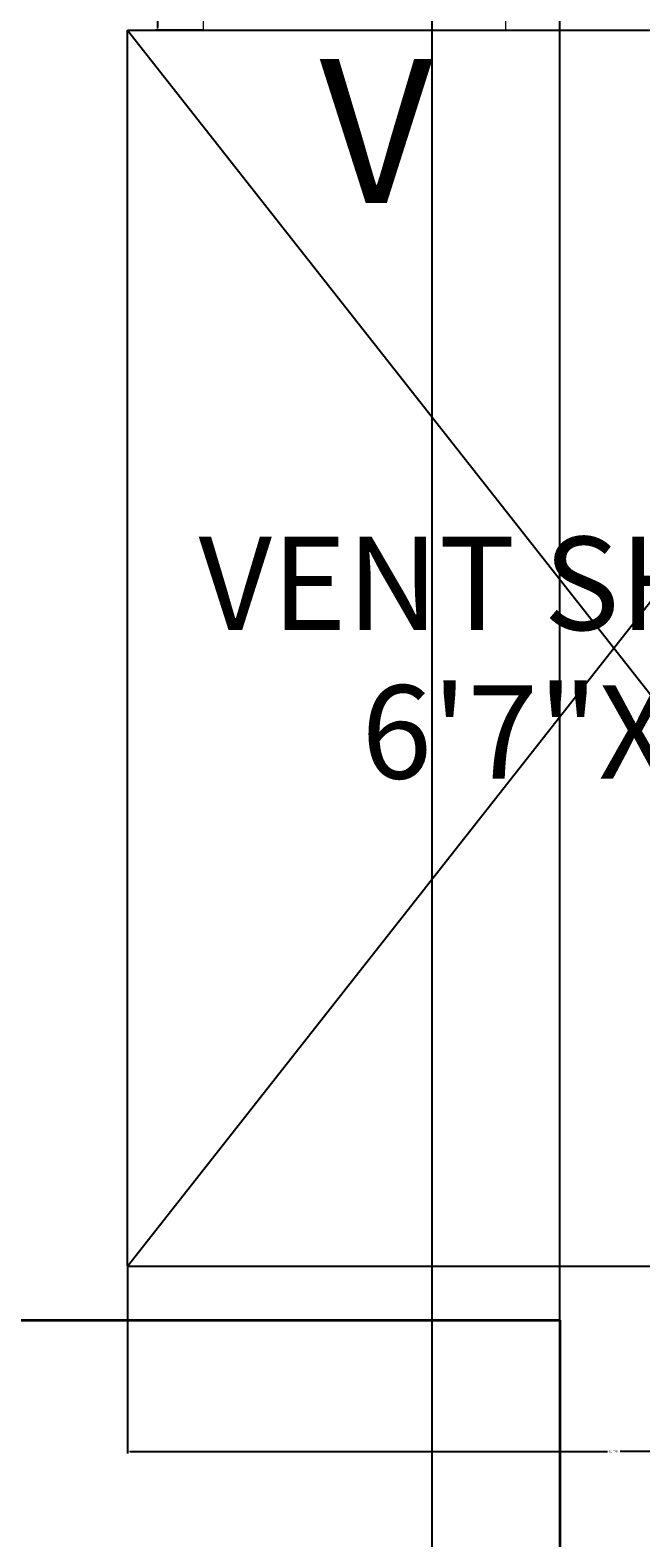
# Model space of a CAD drawing. Units: feet. Extents: x 5816 to 6644, y 25475 to 26788.
# Tile 16 of 23: x 6181 to 6232, y 26373 to 26499. Entities that reach past the tile are written whole.
import ezdxf

# ---------------------------------------------------------------- set-up
doc = ezdxf.new("R2010")
doc.units = ezdxf.units.FT
for name, color, linetype, lineweight in [('A-ANNO-DIMS', 2, 'Continuous', 13), ('A-ANNO-TEXT', 7, 'Continuous', 18), ('A-AREA-IDEN', 7, 'Continuous', 18), ('A-FLOR-SHFT', 8, 'Continuous', 25), ('A-GLAZ', 4, 'Continuous', 18), ('A-WALL', 7, 'Continuous', 35)]:
    doc.layers.add(name, color=color, linetype=linetype, lineweight=lineweight)
doc.styles.get("Standard").update_dxf_attribs({"font": 'arial.ttf'})
doc.dimstyles.get("Standard").update_dxf_attribs({"dimtxt": 0.18, "dimasz": 0.18, "dimexe": 0.18, "dimexo": 0.0625, "dimgap": 0.09, "dimtad": 0, "dimtih": 1, "dimtoh": 1, "dimdec": 4, "dimzin": 0, "dimdsep": 46, "dimtxsty": 'Standard', "dimcen": 0.09, "dimadec": 0, "dimazin": 0, "dimtfac": 1, "dimtdec": 4, "dimtofl": 0, "dimtmove": 0, "dimatfit": 3, "dimfxl": 1, "dimtolj": 1, "dimtzin": 0, "dimarcsym": 0})

# ---------------------------------------------------------------- blocks, each defined once
blk = doc.blocks.new('WIN-VENT-WIDE')
for p, q in [((0, 0), (0, -9)), ((25.2, 0), (25.2, -9)), ((0, -4.5), (25.2, -4.5))]:
    blk.add_line(p, q)
blk = doc.blocks.new('VENT-SHAFT')
for p, q in [((0, 0), (0, 103)), ((0, 103), (81, 103)), ((0, 103), (81, 0)), ((0, 0), (81, 103)), ((81, 103), (45, 103)), ((81, 0), (81, 103)), ((0, 0), (81, 0)), ((81, 0), (45, 0))]:
    blk.add_line(p, q)
blk = doc.blocks.new('*D50')
at = {"layer": 'A-ANNO-DIMS', "color": 0, "lineweight": -2, "transparency": 16777216}
for p, q in [((6195.53, 26507.58), (6191.64, 26507.58)), ((6191.82, 26507.4), (6191.82, 26503.27)), ((6191.82, 26498.76), (6191.82, 26502.9)), ((6195.53, 26498.58), (6191.64, 26498.58))]:
    blk.add_line(p, q, dxfattribs=at)
at = {"layer": 'A-ANNO-DIMS', "color": 0, "transparency": 16777216}
for points in [[(6191.79, 26507.4), (6191.85, 26507.4), (6191.82, 26507.58)], [(6191.79, 26498.76), (6191.85, 26498.76), (6191.82, 26498.58)]]:
    blk.add_solid(points, dxfattribs=at)
at = {"layer": 'Defpoints', "color": 0, "transparency": 16777216}
for p in [(6191.82, 26507.58), (6195.6, 26507.58), (6195.6, 26498.58)]:
    blk.add_point(p, dxfattribs=at)
at = {"layer": 'A-ANNO-DIMS', "color": 0, "transparency": 16777216, "insert": (6191.82, 26503.08), "char_height": 0.18, "attachment_point": 5}
blk.add_mtext('\\A1;9 TYP.', dxfattribs=at)
blk = doc.blocks.new('*D54')
at = {"layer": 'A-ANNO-DIMS', "color": 0, "lineweight": -2, "transparency": 16777216}
for p, q in [((6189.31, 26395.52), (6189.31, 26379.95)), ((6270.31, 26395.52), (6270.31, 26379.95)), ((6189.49, 26380.13), (6229.28, 26380.13)), ((6270.13, 26380.13), (6230.34, 26380.13))]:
    blk.add_line(p, q, dxfattribs=at)
at = {"layer": 'A-ANNO-DIMS', "color": 0, "transparency": 16777216}
for points in [[(6189.49, 26380.16), (6189.49, 26380.1), (6189.31, 26380.13)], [(6270.13, 26380.16), (6270.13, 26380.1), (6270.31, 26380.13)]]:
    blk.add_solid(points, dxfattribs=at)
at = {"layer": 'Defpoints', "color": 0, "transparency": 16777216}
for p in [(6189.31, 26395.58), (6270.31, 26395.58), (6270.31, 26380.13)]:
    blk.add_point(p, dxfattribs=at)
at = {"layer": 'A-ANNO-DIMS', "color": 0, "transparency": 16777216, "insert": (6229.81, 26380.13), "char_height": 0.18, "attachment_point": 5}
blk.add_mtext('\\A1;81 TYP.', dxfattribs=at)
blk = doc.blocks.new('*D60')
at = {"layer": 'A-ANNO-DIMS', "color": 0, "lineweight": -2, "transparency": 16777216}
for p, q in [((6106.98, 26094.4), (6106.98, 26787.91)), ((6107.16, 26787.73), (6224.93, 26787.73)), ((6343.5, 26787.73), (6225.72, 26787.73)), ((6343.68, 26094.4), (6343.68, 26787.91))]:
    blk.add_line(p, q, dxfattribs=at)
at = {"layer": 'A-ANNO-DIMS', "color": 0, "transparency": 16777216}
for points in [[(6107.16, 26787.76), (6107.16, 26787.7), (6106.98, 26787.73)], [(6343.5, 26787.76), (6343.5, 26787.7), (6343.68, 26787.73)]]:
    blk.add_solid(points, dxfattribs=at)
at = {"layer": 'Defpoints', "color": 0, "transparency": 16777216}
for p in [(6343.68, 26787.73), (6106.98, 26094.34), (6343.68, 26094.34)]:
    blk.add_point(p, dxfattribs=at)
at = {"layer": 'A-ANNO-DIMS', "color": 0, "transparency": 16777216, "insert": (6225.33, 26787.73), "char_height": 0.18, "attachment_point": 5}
blk.add_mtext('\\A1;236.7', dxfattribs=at)
blk = doc.blocks.new('*D72')
at = {"layer": 'A-ANNO-DIMS', "color": 0, "lineweight": -2, "transparency": 16777216}
for p, q in [((6214.69, 26168.65), (6214.69, 26787.91)), ((6214.87, 26787.73), (6219.56, 26787.73)), ((6225.13, 26787.73), (6220.44, 26787.73)), ((6225.31, 26177.65), (6225.31, 26787.91))]:
    blk.add_line(p, q, dxfattribs=at)
at = {"layer": 'A-ANNO-DIMS', "color": 0, "transparency": 16777216}
for points in [[(6214.87, 26787.76), (6214.87, 26787.7), (6214.69, 26787.73)], [(6225.13, 26787.76), (6225.13, 26787.7), (6225.31, 26787.73)]]:
    blk.add_solid(points, dxfattribs=at)
at = {"layer": 'Defpoints', "color": 0, "transparency": 16777216}
for p in [(6225.31, 26787.73), (6225.31, 26177.58), (6214.69, 26168.58)]:
    blk.add_point(p, dxfattribs=at)
at = {"layer": 'A-ANNO-DIMS', "color": 0, "transparency": 16777216, "insert": (6220, 26787.73), "char_height": 0.18, "attachment_point": 5}
blk.add_mtext('\\A1;10.621', dxfattribs=at)

msp = doc.modelspace()

# ---------------------------------------------------------------- linework, layer by layer
at = {"layer": 'A-WALL'}
for p, q in [((6123.3119, 26391.0846), (6225.3119, 26391.0846)), ((6225.3119, 26391.0846), (6225.3119, 26177.5846))]:
    msp.add_line(p, q, dxfattribs=at)

# ---------------------------------------------------------------- block references
at = {"layer": 'A-FLOR-SHFT'}
msp.add_blockref('VENT-SHAFT', (6189.3119, 26395.5846), dxfattribs=at)
at = {"layer": 'A-GLAZ'}
msp.add_blockref('WIN-VENT-WIDE', (6195.5951, 26507.5846), dxfattribs=at)

# ---------------------------------------------------------------- texts
at = {"layer": 'A-ANNO-DIMS'}
msp.add_text('6\'7"X8\'2"', height=7.77416, dxfattribs=at).set_placement((6208.7805, 26436.2088))
at = {"layer": 'A-ANNO-TEXT'}
msp.add_text('V', height=12, dxfattribs=at).set_placement((6205.3013, 26484.1731))
at = {"layer": 'A-AREA-IDEN'}
msp.add_text('VENT SHAFT', height=7.77416, dxfattribs=at).set_placement((6195.225, 26448.5899))

# ---------------------------------------------------------------- dimensions: what is measured, and where the dimension line sits
at = {"layer": 'A-ANNO-DIMS'}
for base, p1, p2, override, picture, middle in [((6343.6763, 26787.7346), (6106.9781, 26094.3368), (6343.6763, 26094.3368), {"dimdec": 1, "dimlfac": 1, "dimrnd": 0, "dimzin": 0, "dimdsep": 46, "dimlunit": 2}, '*D60', (6225.3272, 26787.7346)), ((6225.3119, 26787.7346), (6214.6905, 26168.5846), (6225.3119, 26177.5846), {"dimdec": 3, "dimlfac": 1, "dimrnd": 0, "dimzin": 0, "dimdsep": 46, "dimlunit": 2}, '*D72', (6220.0012, 26787.7346))]:
    dim = msp.add_linear_dim(base=base, p1=p1, p2=p2, dimstyle='Standard', override=override, dxfattribs=at)
    dim.commit()
    dim.dimension.update_dxf_attribs({"geometry": picture, "text_midpoint": middle})
dim = msp.add_linear_dim(base=(6191.8152, 26507.5846), p1=(6195.5951, 26498.5846), p2=(6195.5951, 26507.5846), angle=90, text='<> TYP.', dimstyle='Standard', override={"dimdec": 0, "dimlfac": 1, "dimrnd": 0, "dimzin": 0, "dimdsep": 46, "dimlunit": 2}, dxfattribs=at)
dim.commit()
dim.dimension.update_dxf_attribs({"geometry": '*D50', "text_midpoint": (6191.8152, 26503.0846)})
dim = msp.add_linear_dim(base=(6270.3119, 26380.1346), p1=(6189.3119, 26395.5846), p2=(6270.3119, 26395.5846), text='<> TYP.', dimstyle='Standard', override={"dimdec": 0, "dimlfac": 1, "dimrnd": 0, "dimzin": 0, "dimdsep": 46, "dimlunit": 2}, dxfattribs=at)
dim.commit()
dim.dimension.update_dxf_attribs({"geometry": '*D54', "text_midpoint": (6229.8119, 26380.1346)})

doc.saveas('drawing.dxf')
